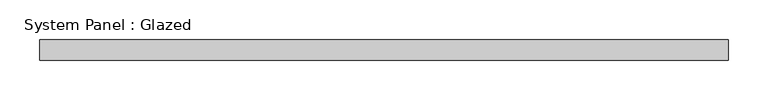
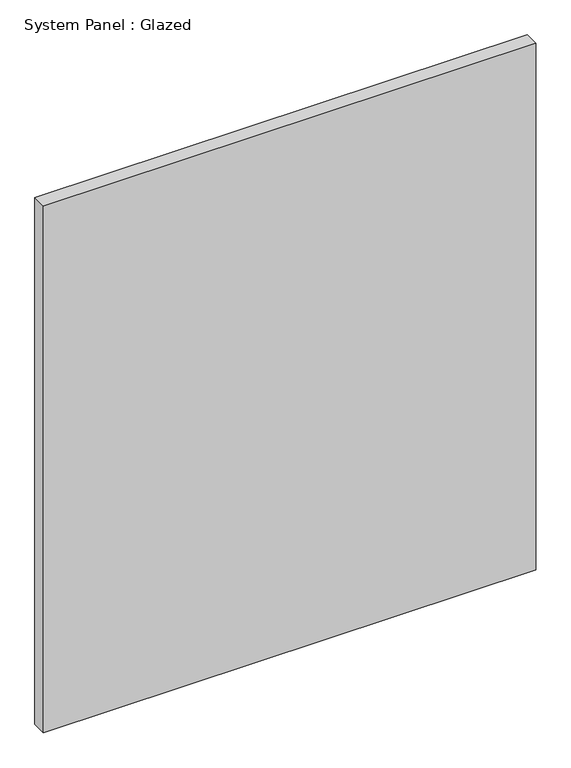
"""IFC4 building model written with IfcOpenShell, lengths in millimetres: plate geometry, System Panel : Glazed."""

from ifc_helpers import new_model, si_unit, origin, origin_with_axes, place, context, project, spatial, polyline, outline, extrude, source, transform, mapped, element, save


def system_panel_glazed_ee4e9f01(model_context):
    return source(origin(), model_context, "Body", "SweptSolid", [
        extrude(outline(polyline([(432.3220098, 19.05), (-432.3220098, 19.05), (-432.3220098, 44.45), (432.3220098, 44.45), (432.3220098, 19.05)])), origin_with_axes(), (0.0, 0.0, 1.0), 977.9),
    ])


if __name__ == "__main__":
    model = new_model("IFC4")
    model_context = context("Model", 3, world=origin())
    ifc_project = project(units=[si_unit("LENGTHUNIT", "METRE", prefix="MILLI")], contexts=[model_context])
    site = spatial("IfcSite", under=ifc_project)
    building = spatial("IfcBuilding", under=site)
    placement = place(None, origin())
    system_panel_glazed_shape = system_panel_glazed_ee4e9f01(model_context)
    element("IfcPlate", 1, ObjectType="System Panel : Glazed", at=placement, inside=building, context=model_context, shape_type="MappedRepresentation", body=[
        mapped(system_panel_glazed_shape, transform((0.0, 0.0, 0.0), x_axis=(1.0, 0.0, 0.0), y_axis=(0.0, 1.0, 0.0), z_axis=(0.0, 0.0, 1.0))),
    ])
    save(model, "model.ifc")

# Revit data of these elements
# Type "System Panel : Glazed"
#   Construction Type Id = "GSP4R"
#   Analytic Construction = "1/8 in Pilkington single glazing"
#   Visual Light Transmittance = 0.9
#   Solar Heat Gain Coefficient = 0.86
#   Heat Transfer Coefficient (U) = 1.18115 BTU/(h·ft²·°F)
#   Define Thermal Properties by = 1
# Element 1 (IfcPlate, "System Panel : Glazed")
#   Materials on its faces: "Glass"
# Materials
#   "Glass": class "Glass", colour RGB 0 128 192, transparency 0.75, Description = "Soda Lime Glass", Cost = 0
